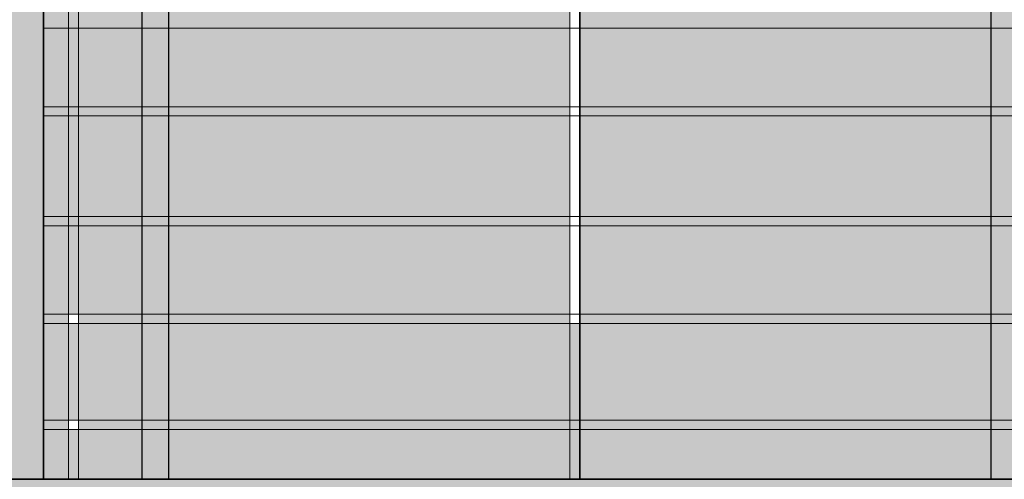
# Model space of a CAD drawing. Units: feet. Extents: x 2695 to 2912, y 795 to 1139.
# Tile 52 of 83: x 2769 to 2843, y 937 to 971. Entities that reach past the tile are written whole.
import ezdxf

# ---------------------------------------------------------------- set-up
doc = ezdxf.new("R2010")
doc.units = ezdxf.units.FT
for name, color, linetype, lineweight in [('A-ELEV', 7, 'Continuous', 35), ('A-ELEV-PATT', 252, 'Continuous', 13), ('A-ELEV-RAIL', 8, 'Continuous', 18), ('A-GLAZ', 4, 'Continuous', 25), ('A-GLAZ-PATT', 254, 'Continuous', 13)]:
    doc.layers.add(name, color=color, linetype=linetype, lineweight=lineweight)

msp = doc.modelspace()

# ---------------------------------------------------------------- hatches: boundary and pattern name
at = {"layer": 'A-ELEV-PATT'}
h = msp.add_hatch(color=256, dxfattribs=at)
h.set_gradient(color1=(255, 255, 255), tint=1)
h.paths.add_polyline_path([(2770.6361, 1122.9306), (2710.6361, 1122.9306), (2710.6361, 1118.4096), (2770.6361, 1118.4096)])
h.paths.add_polyline_path([(2890.6361, 1107.8588), (2770.6361, 1107.8588), (2770.6361, 1103.3378), (2890.6361, 1103.3378)])
h.paths.add_polyline_path([(2890.6361, 1062.9306), (2710.6361, 1062.9306), (2710.6361, 1056.9306), (2710.6361, 936.9306), (2710.6361, 924.3105), (2716.5358, 924.3105), (2890.6361, 924.3105), (2890.6361, 936.9306), (2715.8852, 936.9306), (2715.8852, 1050.3105), (2890.6361, 1050.3105)])
h.paths.add_polyline_path([(2716.5358, 924.3105), (2710.6361, 924.3105), (2710.6361, 810.9306), (2716.5358, 810.9306)])
h = msp.add_hatch(color=256, dxfattribs=at)
h.set_gradient(color1=(147, 149, 152), color2=(147, 149, 152), tint=1)
h.paths.add_polyline_path([(2770.6361, 1118.4096), (2710.6361, 1118.4096), (2710.6361, 1062.9306), (2770.6361, 1062.9306)])
h.paths.add_polyline_path([(2890.6361, 1103.3378), (2770.6361, 1103.3378), (2770.6361, 1062.9306), (2890.6361, 1062.9306)])
h.paths.add_polyline_path([(2730.7081, 1048.1052), (2755.1125, 1048.1052), (2755.1125, 936.9306), (2770.6361, 936.9306), (2770.6361, 1050.3105), (2715.8852, 1050.3105), (2715.8852, 936.9306), (2730.7081, 936.9306)])
h.paths.add_polyline_path([(2890.6361, 1050.3105), (2770.6361, 1050.3105), (2770.6361, 971.9673), (2778.0341, 971.9673), (2778.0341, 1020.8235), (2843.575, 1020.8235), (2843.575, 971.9673), (2890.6361, 971.9673)])
h.paths.add_polyline_path([(2888.1882, 970.7156), (2843.575, 970.7156), (2843.575, 964.8267), (2888.1882, 964.8267)])
h.paths.add_polyline_path([(2888.1882, 964.1328), (2843.575, 964.1328), (2843.575, 956.614), (2888.1882, 956.614)])
h.paths.add_polyline_path([(2888.1882, 955.9202), (2843.575, 955.9202), (2843.575, 949.2892), (2888.1882, 949.2892)])
h.paths.add_polyline_path([(2888.1882, 948.5954), (2843.575, 948.5954), (2843.575, 941.3507), (2888.1882, 941.3507)])
h.paths.add_polyline_path([(2888.1882, 940.6569), (2843.575, 940.6569), (2843.575, 936.9306), (2888.1882, 936.9306)])
h.paths.add_polyline_path([(2890.6361, 970.7156), (2888.9368, 970.7156), (2888.9368, 964.8267), (2890.6361, 964.8267)])
h.paths.add_polyline_path([(2890.6361, 964.1328), (2888.9368, 964.1328), (2888.9368, 956.614), (2890.6361, 956.614)])
h.paths.add_polyline_path([(2890.6361, 955.9202), (2888.9368, 955.9202), (2888.9368, 949.2892), (2890.6361, 949.2892)])
h.paths.add_polyline_path([(2890.6361, 940.6569), (2888.9368, 940.6569), (2888.9368, 936.9306), (2890.6361, 936.9306)])
h.paths.add_polyline_path([(2890.6361, 948.5954), (2888.9368, 948.5954), (2888.9368, 941.3507), (2890.6361, 941.3507)])
h.paths.add_polyline_path([(2772.5216, 970.7156), (2770.6361, 970.7156), (2770.6361, 964.8267), (2772.5216, 964.8267)])
h.paths.add_polyline_path([(2772.5216, 964.1328), (2770.6361, 964.1328), (2770.6361, 956.614), (2772.5216, 956.614)])
h.paths.add_polyline_path([(2772.5216, 955.9202), (2770.6361, 955.9202), (2770.6361, 949.2892), (2772.5216, 949.2892)])
h.paths.add_polyline_path([(2772.5216, 948.5954), (2770.6361, 948.5954), (2770.6361, 941.3507), (2772.5216, 941.3507)])
h.paths.add_polyline_path([(2772.5216, 940.6569), (2770.6361, 940.6569), (2770.6361, 936.9306), (2772.5216, 936.9306)])
h.paths.add_polyline_path([(2778.0341, 940.6569), (2773.2702, 940.6569), (2773.2702, 936.9306), (2778.0341, 936.9306)])
h.paths.add_polyline_path([(2778.0341, 970.7156), (2773.2702, 970.7156), (2773.2702, 964.8267), (2778.0341, 964.8267)])
h.paths.add_polyline_path([(2778.0341, 964.1328), (2773.2702, 964.1328), (2773.2702, 956.614), (2778.0341, 956.614)])
h.paths.add_polyline_path([(2778.0341, 955.9202), (2773.2702, 955.9202), (2773.2702, 949.2892), (2778.0341, 949.2892)])
h.paths.add_polyline_path([(2778.0341, 948.5954), (2773.2702, 948.5954), (2773.2702, 941.3507), (2778.0341, 941.3507)])
h.paths.add_polyline_path([(2810.0407, 940.6569), (2780.0341, 940.6569), (2780.0341, 936.9306), (2810.0407, 936.9306)])
h.paths.add_polyline_path([(2890.6361, 924.3105), (2770.6361, 924.3105), (2770.6361, 810.9306), (2773.5029, 810.9306), (2773.5029, 905.5143), (2805.9398, 905.5143), (2838.3767, 905.5143), (2838.3767, 810.9306), (2890.6361, 810.9306)])
h = msp.add_hatch(color=256, dxfattribs=at)
h.set_gradient(color2=(0, 0, 0), tint=1)
h.paths.add_polyline_path([(2772.5216, 971.9673), (2770.6361, 971.9673), (2770.6361, 970.7156), (2772.5216, 970.7156)])
h.paths.add_polyline_path([(2773.2702, 971.9673), (2772.5216, 971.9673), (2772.5216, 970.7156), (2773.2702, 970.7156)])
h.paths.add_polyline_path([(2778.0341, 971.9673), (2773.2702, 971.9673), (2773.2702, 970.7156), (2778.0341, 970.7156)])
h.paths.add_polyline_path([(2780.0341, 971.9673), (2778.0341, 971.9673), (2778.0341, 970.7156), (2780.0341, 970.7156)])
h.paths.add_polyline_path([(2841.575, 971.9673), (2780.0341, 971.9673), (2780.0341, 970.7156), (2841.575, 970.7156)])
h.paths.add_polyline_path([(2843.575, 971.9673), (2841.575, 971.9673), (2841.575, 970.7156), (2843.575, 970.7156)])
h.paths.add_polyline_path([(2888.1882, 971.9673), (2843.575, 971.9673), (2843.575, 970.7156), (2888.1882, 970.7156)])
h.paths.add_polyline_path([(2888.9368, 971.9673), (2888.1882, 971.9673), (2888.1882, 970.7156), (2888.9368, 970.7156)], flags=17)
h.paths.add_polyline_path([(2890.6361, 971.9673), (2888.9368, 971.9673), (2888.9368, 970.7156), (2890.6361, 970.7156)])
h.paths.add_polyline_path([(2888.9368, 971.9673), (2888.1882, 971.9673), (2888.1882, 964.8267), (2888.9368, 964.8267)])
h.paths.add_polyline_path([(2888.9368, 964.8267), (2888.1882, 964.8267), (2888.1882, 964.1328), (2888.9368, 964.1328)])
h.paths.add_polyline_path([(2890.6361, 964.8267), (2888.9368, 964.8267), (2888.9368, 964.1328), (2890.6361, 964.1328)])
h.paths.add_polyline_path([(2888.1882, 964.8267), (2770.6361, 964.8267), (2770.6361, 964.1328), (2888.1882, 964.1328)])
h.paths.add_polyline_path([(2888.9368, 964.1328), (2888.1882, 964.1328), (2888.1882, 936.9306), (2888.9368, 936.9306)])
h.paths.add_polyline_path([(2890.6361, 956.614), (2888.9368, 956.614), (2888.9368, 955.9202), (2890.6361, 955.9202)])
h.paths.add_polyline_path([(2888.1882, 956.614), (2770.6361, 956.614), (2770.6361, 955.9202), (2888.1882, 955.9202)])
h.paths.add_polyline_path([(2890.6361, 949.2892), (2888.9368, 949.2892), (2888.9368, 948.5954), (2890.6361, 948.5954)])
h.paths.add_polyline_path([(2888.1882, 949.2892), (2770.6361, 949.2892), (2770.6361, 948.5954), (2888.1882, 948.5954)])
h.paths.add_polyline_path([(2890.6361, 941.3507), (2888.9368, 941.3507), (2888.9368, 940.6569), (2890.6361, 940.6569)])
h.paths.add_polyline_path([(2888.1882, 941.3507), (2770.6361, 941.3507), (2770.6361, 940.6569), (2888.1882, 940.6569)])
h.paths.add_polyline_path([(2773.2702, 970.7156), (2772.5216, 970.7156), (2772.5216, 964.8267), (2773.2702, 964.8267)])
h.paths.add_polyline_path([(2773.2702, 964.1328), (2772.5216, 964.1328), (2772.5216, 956.614), (2773.2702, 956.614)])
h.paths.add_polyline_path([(2773.2702, 955.9202), (2772.5216, 955.9202), (2772.5216, 936.9306), (2773.2702, 936.9306)])
h.paths.add_polyline_path([(2810.7893, 970.7156), (2810.0407, 970.7156), (2810.0407, 964.8267), (2810.7893, 964.8267)], flags=17)
h.paths.add_polyline_path([(2810.7893, 964.1328), (2810.0407, 964.1328), (2810.0407, 956.614), (2810.7893, 956.614)], flags=17)
h.paths.add_polyline_path([(2810.7893, 955.9202), (2810.0407, 955.9202), (2810.0407, 949.2892), (2810.7893, 949.2892)], flags=17)
h.paths.add_polyline_path([(2810.7893, 971.9673), (2810.0407, 971.9673), (2810.0407, 941.3507), (2810.7893, 941.3507)])
h.paths.add_polyline_path([(2810.7893, 940.6569), (2810.0407, 940.6569), (2810.0407, 936.9306), (2810.7893, 936.9306)])
h.paths.add_polyline_path([(2780.0341, 1018.8235), (2841.575, 1018.8235), (2841.575, 971.9673), (2843.575, 971.9673), (2843.575, 1020.8235), (2778.0341, 1020.8235), (2778.0341, 971.9673), (2780.0341, 971.9673)])
h.paths.add_polyline_path([(2780.0341, 970.7156), (2778.0341, 970.7156), (2778.0341, 964.8267), (2780.0341, 964.8267)])
h.paths.add_polyline_path([(2780.0341, 964.1328), (2778.0341, 964.1328), (2778.0341, 956.614), (2780.0341, 956.614)])
h.paths.add_polyline_path([(2780.0341, 955.9202), (2778.0341, 955.9202), (2778.0341, 949.2892), (2780.0341, 949.2892)])
h.paths.add_polyline_path([(2780.0341, 948.5954), (2778.0341, 948.5954), (2778.0341, 941.3507), (2780.0341, 941.3507)])
h.paths.add_polyline_path([(2780.0341, 940.6569), (2778.0341, 940.6569), (2778.0341, 936.9306), (2780.0341, 936.9306)])
h.paths.add_polyline_path([(2843.575, 940.6569), (2841.575, 940.6569), (2841.575, 936.9306), (2843.575, 936.9306)])
h.paths.add_polyline_path([(2843.575, 948.5954), (2841.575, 948.5954), (2841.575, 941.3507), (2843.575, 941.3507)])
h.paths.add_polyline_path([(2843.575, 970.7156), (2841.575, 970.7156), (2841.575, 964.8267), (2843.575, 964.8267)])
h.paths.add_polyline_path([(2843.575, 964.1328), (2841.575, 964.1328), (2841.575, 956.614), (2843.575, 956.614)])
h.paths.add_polyline_path([(2843.575, 955.9202), (2841.575, 955.9202), (2841.575, 949.2892), (2843.575, 949.2892)])
h.paths.add_polyline_path([(2805.0538, 874.1057), (2803.9681, 874.1057), (2803.9681, 846.2857), (2805.0538, 846.2857)])
h.paths.add_polyline_path([(2758.1515, 902.577), (2724.1893, 902.577), (2724.1893, 874.8571), (2758.1515, 874.8571)])
h.paths.add_polyline_path([(2726.1893, 900.577), (2756.1515, 900.577), (2756.1515, 876.8571), (2726.1893, 876.8571)], flags=16)
h.paths.add_polyline_path([(2740.7302, 900.577), (2741.6105, 900.577), (2741.6105, 876.8571), (2740.7302, 876.8571)], flags=0)
at = {"layer": 'A-GLAZ-PATT'}
h = msp.add_hatch(color=256, dxfattribs=at)
h.set_gradient(color1=(213, 227, 240), color2=(213, 227, 240))
h.paths.add_polyline_path([(2810.8045, 1018.8235), (2780.0341, 1018.8235), (2780.0341, 971.9673), (2810.8045, 971.9673)])
h.paths.add_polyline_path([(2841.575, 1018.8235), (2810.8045, 1018.8235), (2810.8045, 971.9673), (2841.575, 971.9673)])
h.paths.add_polyline_path([(2810.0407, 970.7156), (2780.0341, 970.7156), (2780.0341, 964.8267), (2810.0407, 964.8267)])
h.paths.add_polyline_path([(2841.575, 970.7156), (2810.8045, 970.7156), (2810.8045, 964.8267), (2841.575, 964.8267)])
h.paths.add_polyline_path([(2841.575, 964.1328), (2810.8045, 964.1328), (2810.8045, 956.614), (2841.575, 956.614)])
h.paths.add_polyline_path([(2810.0407, 964.1328), (2780.0341, 964.1328), (2780.0341, 956.614), (2810.0407, 956.614)])
h.paths.add_polyline_path([(2810.0407, 955.9202), (2780.0341, 955.9202), (2780.0341, 949.2892), (2810.0407, 949.2892)])
h.paths.add_polyline_path([(2841.575, 955.9202), (2810.8045, 955.9202), (2810.8045, 949.2892), (2841.575, 949.2892)])
h.paths.add_polyline_path([(2841.575, 948.5954), (2810.8045, 948.5954), (2810.8045, 941.3507), (2841.575, 941.3507)])
h.paths.add_polyline_path([(2810.0407, 948.5954), (2780.0341, 948.5954), (2780.0341, 941.3507), (2810.0407, 941.3507)])
h.paths.add_polyline_path([(2810.0407, 940.6569), (2780.0341, 940.6569), (2780.0341, 936.9306), (2810.0407, 936.9306)])
h.paths.add_polyline_path([(2841.575, 940.6569), (2810.8045, 940.6569), (2810.8045, 936.9306), (2841.575, 936.9306)])

# ---------------------------------------------------------------- linework, layer by layer
at = {"layer": 'A-ELEV'}
for p, q in [((2770.6361, 1050.3105), (2770.6361, 936.9306)), ((2715.8852, 936.9306), (2890.6361, 936.9306)), ((2715.8852, 936.9306), (2890.6361, 936.9306))]:
    msp.add_line(p, q, dxfattribs=at)
at = {"layer": 'A-ELEV-RAIL'}
for points in [[(2773.2702, 971.9673), (2772.5216, 971.9673), (2772.5216, 936.9306), (2773.2702, 936.9306)], [(2810.7893, 971.9673), (2810.0407, 971.9673), (2810.0407, 936.9306), (2810.7893, 936.9306)], [(2770.6361, 964.1328), (2890.6361, 964.1328), (2890.6361, 964.8267), (2770.6361, 964.8267)], [(2770.6361, 955.9202), (2890.6361, 955.9202), (2890.6361, 956.614), (2770.6361, 956.614)], [(2770.6361, 948.5954), (2890.6361, 948.5954), (2890.6361, 949.2892), (2770.6361, 949.2892)], [(2770.6361, 940.6569), (2890.6361, 940.6569), (2890.6361, 941.3507), (2770.6361, 941.3507)]]:
    msp.add_lwpolyline(points, close=True, dxfattribs=at)
msp.add_lwpolyline([(2770.6361, 970.7156), (2890.6361, 970.7156)], dxfattribs=at)
at = {"layer": 'A-GLAZ'}
for points in [[(2778.0341, 936.9306), (2778.0341, 1020.8235), (2843.575, 1020.8235), (2843.575, 936.9306)], [(2780.0341, 936.9306), (2780.0341, 1018.8235), (2841.575, 1018.8235), (2841.575, 936.9306)]]:
    msp.add_lwpolyline(points, dxfattribs=at)
for points in [[(2810.8045, 1018.8235), (2810.7893, 1018.8235), (2810.7893, 936.9306), (2810.8045, 936.9306)], [(2810.8045, 1018.8235), (2810.8045, 1018.8235), (2810.8045, 936.9306), (2810.8045, 936.9306)]]:
    msp.add_lwpolyline(points, close=True, dxfattribs=at)

doc.saveas('drawing.dxf')
